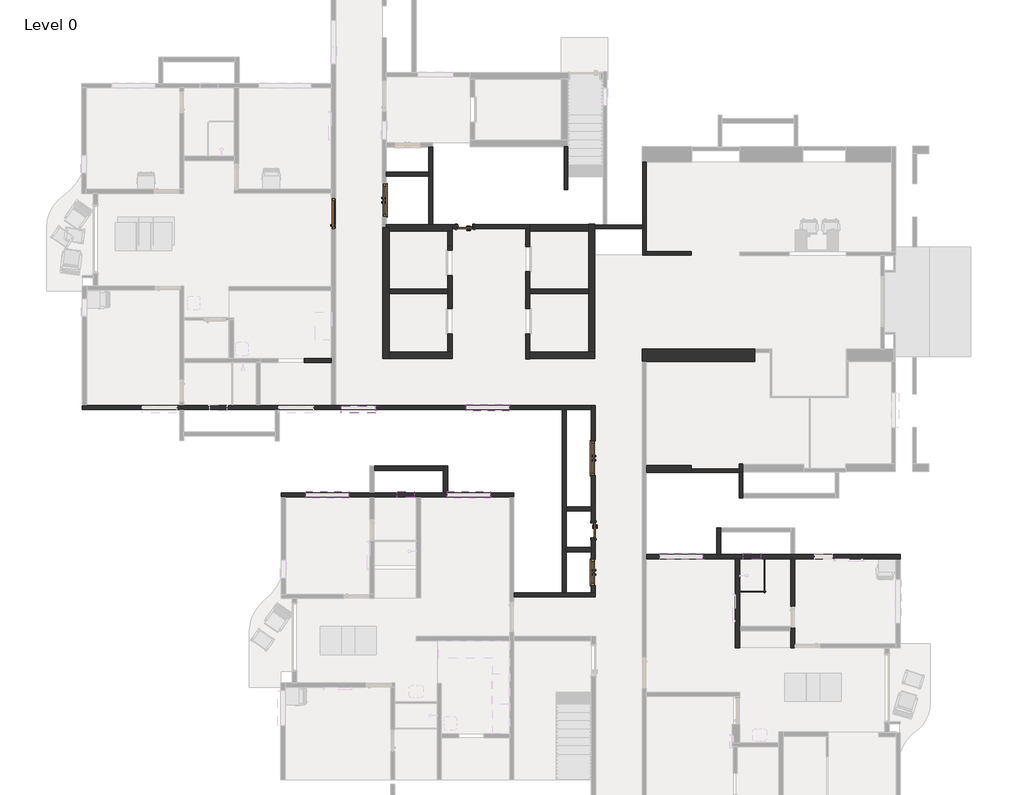
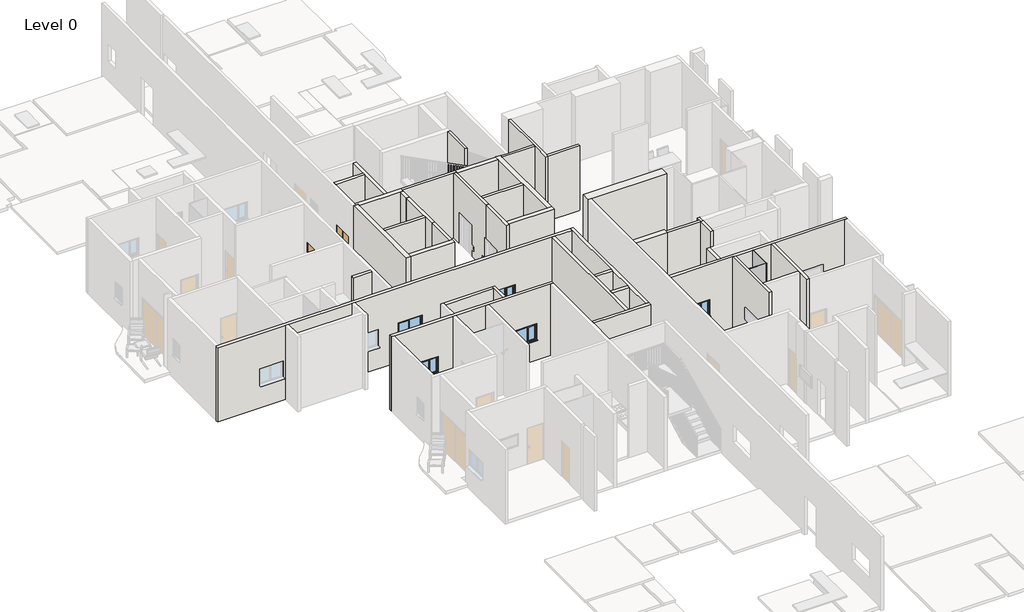
# One storey, part 5 of 14: 39 walls, 7 windows, 6 doors, 2 plates.
"""IFC4 building model written with IfcOpenShell, lengths in millimetres."""

from ifc_helpers import new_model, si_unit, origin, origin_with_axes, place, context, project, spatial, polyline, outline, extrude, faceted_brep, transform, mapped, element, save
from components import doors_extdbl_flush_3_b8e651f3, doors_extdbl_flush_3_75_39ca422f, doors_extdbl_flush_4_40db91a8, doors_extsgl_flush_d1_30a970b5, doors_intsgl_2_0e89f101, system_panel_glazed_234dce3e, system_panel_glazed_3e513c0f, windows_concept_plain_dbl_4_d1e2e333, windows_sgl_plain_2_be143095, windows_tpl_variable_casement_5_ffad3fa3

model = new_model("IFC4")

# Units and contexts
model_context = context("Model", 3, world=origin())
ifc_project = project(units=[si_unit("LENGTHUNIT", "METRE", prefix="MILLI")], contexts=[model_context])

# Site, building, storey
site = spatial("IfcSite", under=ifc_project)
building = spatial("IfcBuilding", under=site)
storey = spatial("IfcBuildingStorey", under=building, Name="Level 0", Elevation=0.0)

# Doors
placement = place(None, origin())
doors_extdbl_flush_3_shape = doors_extdbl_flush_3_b8e651f3(model_context)
element("IfcDoor", 1, ObjectType="Doors_ExtDbl_Flush : 3'", at=placement, inside=storey, context=model_context, shape_type="MappedRepresentation", body=[
    mapped(doors_extdbl_flush_3_shape, transform((-21675.1800447, 33308.7351384, 0.0), x_axis=(0.0, 1.0, 0.0), y_axis=(-1.0, 0.0, 0.0), z_axis=(0.0, 0.0, 1.0))),
])
doors_extdbl_flush_3_75_shape = doors_extdbl_flush_3_75_39ca422f(model_context)
element("IfcDoor", 2, ObjectType="Doors_ExtDbl_Flush : 3.75'", at=placement, inside=storey, context=model_context, shape_type="MappedRepresentation", body=[
    mapped(doors_extdbl_flush_3_75_shape, transform((-29094.6788109, 46525.3706597, 0.0), x_axis=(0.0, -1.0, 0.0), y_axis=(1.0, 0.0, 0.0), z_axis=(0.0, 0.0, 1.0))),
])
doors_extdbl_flush_4_shape = doors_extdbl_flush_4_40db91a8(model_context)
element("IfcDoor", 3, ObjectType="Doors_ExtDbl_Flush : 4'", at=placement, inside=storey, context=model_context, shape_type="MappedRepresentation", body=[
    mapped(doors_extdbl_flush_4_shape, transform((-21675.1800447, 37361.9567572, 0.0), x_axis=(0.0, 1.0, 0.0), y_axis=(-1.0, 0.0, 0.0), z_axis=(0.0, 0.0, 1.0))),
])
doors_extsgl_flush_d1_shape = doors_extsgl_flush_d1_30a970b5(model_context)
element("IfcDoor", 4, ObjectType="Doors_ExtSgl_Flush : D1", at=placement, inside=storey, context=model_context, shape_type="MappedRepresentation", body=[
    mapped(doors_extsgl_flush_d1_shape, transform((-30896.1442282, 46044.6966557, 0.0), x_axis=(0.0, 1.0, 0.0), y_axis=(-1.0, 0.0, 0.0), z_axis=(0.0, 0.0, 1.0))),
])
doors_intsgl_2_shape = doors_intsgl_2_0e89f101(model_context)
element("IfcDoor", 5, ObjectType="Doors_IntSgl : 2'", at=placement, inside=storey, context=model_context, shape_type="MappedRepresentation", body=[
    mapped(doors_intsgl_2_shape, transform((-21675.1800447, 34796.5704211, 0.0), x_axis=(0.0, -1.0, 0.0), y_axis=(1.0, 0.0, 0.0), z_axis=(0.0, 0.0, 1.0))),
])
element("IfcDoor", 6, ObjectType="Doors_IntSgl : 2'", at=placement, inside=storey, context=model_context, shape_type="MappedRepresentation", body=[
    mapped(doors_intsgl_2_shape, transform((-26226.4805211, 45585.4690597, 0.0), x_axis=(-1.0, 0.0, 0.0), y_axis=(0.0, -1.0, 0.0), z_axis=(0.0, 0.0, 1.0))),
])

# Plates
system_panel_glazed_shape = system_panel_glazed_234dce3e(model_context)
element("IfcPlate", 7, ObjectType="System Panel : Glazed", at=placement, inside=storey, context=model_context, shape_type="MappedRepresentation", body=[
    mapped(system_panel_glazed_shape, transform((-16019.2486976, 32586.7114683, 0.0), x_axis=(1.0, 0.0, 0.0), y_axis=(0.0, 1.0, 0.0), z_axis=(0.0, 0.0, 1.0))),
])
system_panel_glazed_2_shape = system_panel_glazed_3e513c0f(model_context)
element("IfcPlate", 8, ObjectType="System Panel : Glazed", at=placement, inside=storey, context=model_context, shape_type="MappedRepresentation", body=[
    mapped(system_panel_glazed_2_shape, transform((-15562.0486976, 33186.8118683, 0.0), x_axis=(0.0, 1.0, 0.0), y_axis=(-1.0, 0.0, 0.0), z_axis=(0.0, 0.0, 1.0))),
])

# Walls
element("IfcWall", 9, ObjectType="W1", at=placement, inside=storey, context=model_context, shape_type="Brep", body=[
    faceted_brep([(-24494.5800447, 36137.3800488, 0.0), (-26841.4029681, 36137.3800488, 0.0), (-26993.8029681, 36137.3800488, 0.0), (-29458.4489269, 36137.3800488, 0.0), (-29610.8489269, 36137.3800488, 0.0), (-32744.0041796, 36137.3800488, 0.0), (-32744.0041796, 36137.3800488, 4000.0), (-29610.8489269, 36137.3800488, 4000.0), (-29458.4489269, 36137.3800488, 4000.0), (-26993.8029681, 36137.3800488, 4000.0), (-26841.4029681, 36137.3800488, 4000.0), (-24494.5800447, 36137.3800488, 4000.0), (-26856.7800447, 36137.3800488, 2110.0), (-26856.7800447, 36137.3800488, 1200.0), (-25332.7800447, 36137.3800488, 1200.0), (-25332.7800447, 36137.3800488, 2110.0), (-31880.4041796, 36137.3800488, 2110.0), (-31880.4041796, 36137.3800488, 1200.0), (-30356.4041796, 36137.3800488, 1200.0), (-30356.4041796, 36137.3800488, 2110.0), (-28638.8447747, 36137.3800488, 2738.9328), (-28638.8447747, 36137.3800488, 1828.9328), (-28029.2447747, 36137.3800488, 1828.9328), (-28029.2447747, 36137.3800488, 2738.9328), (-24494.5800447, 35984.9800488, 0.0), (-24494.5800447, 35984.9800488, 4000.0), (-24646.9800447, 35984.9800488, 4000.0), (-27800.6447747, 35984.9800488, 4000.0), (-27953.0447747, 35984.9800488, 4000.0), (-29458.4489269, 35984.9800488, 4000.0), (-29610.8489269, 35984.9800488, 4000.0), (-32591.6041796, 35984.9800488, 4000.0), (-32744.0041796, 35984.9800488, 4000.0), (-32744.0041796, 35984.9800488, 0.0), (-32591.6041796, 35984.9800488, 0.0), (-29610.8489269, 35984.9800488, 0.0), (-29458.4489269, 35984.9800488, 0.0), (-27953.0447747, 35984.9800488, 0.0), (-27800.6447747, 35984.9800488, 0.0), (-24646.9800447, 35984.9800488, 0.0), (-26856.7800447, 35984.9800488, 2110.0), (-25332.7800447, 35984.9800488, 2110.0), (-25332.7800447, 35984.9800488, 1200.0), (-26856.7800447, 35984.9800488, 1200.0), (-31880.4041796, 35984.9800488, 2110.0), (-30356.4041796, 35984.9800488, 2110.0), (-30356.4041796, 35984.9800488, 1200.0), (-31880.4041796, 35984.9800488, 1200.0), (-28638.8447747, 35984.9800488, 2738.9328), (-28029.2447747, 35984.9800488, 2738.9328), (-28029.2447747, 35984.9800488, 1828.9328), (-28638.8447747, 35984.9800488, 1828.9328)], [[[0, 1, 2, 3, 4, 5, 6, 7, 8, 9, 10, 11], [12, 13, 14, 15], [16, 17, 18, 19], [20, 21, 22, 23]], [[24, 25, 26, 27, 28, 29, 30, 31, 32, 33, 34, 35, 36, 37, 38, 39], [40, 41, 42, 43], [44, 45, 46, 47], [48, 49, 50, 51]], [[5, 4, 3, 2, 1, 0, 24, 39, 38, 37, 36, 35, 34, 33]], [[11, 10, 9, 8, 7, 6, 32, 31, 30, 29, 28, 27, 26, 25]], [[6, 5, 33, 32]], [[0, 11, 25, 24]], [[13, 12, 40, 43]], [[14, 13, 43, 42]], [[15, 14, 42, 41]], [[12, 15, 41, 40]], [[17, 16, 44, 47]], [[18, 17, 47, 46]], [[19, 18, 46, 45]], [[16, 19, 45, 44]], [[21, 20, 48, 51]], [[22, 21, 51, 50]], [[23, 22, 50, 49]], [[20, 23, 49, 48]]]),
])
element("IfcWall", 10, ObjectType="W1", at=placement, inside=storey, context=model_context, shape_type="Brep", body=[
    faceted_brep([(-19793.4917798, 33786.9122683, 0.0), (-16628.8486976, 33786.9122683, 0.0), (-16476.4486976, 33786.9122683, 0.0), (-14673.0486976, 33786.9122683, 0.0), (-14520.6486976, 33786.9122683, 0.0), (-10935.2417798, 33786.9122683, 0.0), (-10782.8417798, 33786.9122683, 0.0), (-10782.8417798, 33786.9122683, 4000.0), (-10935.2417798, 33786.9122683, 4000.0), (-14520.6486976, 33786.9122683, 4000.0), (-14673.0486976, 33786.9122683, 4000.0), (-16476.4486976, 33786.9122683, 4000.0), (-16628.8486976, 33786.9122683, 4000.0), (-19793.4917798, 33786.9122683, 4000.0), (-19309.7710387, 33786.9122683, 2110.0), (-17785.7710387, 33786.9122683, 2110.0), (-17785.7710387, 33786.9122683, 1200.0), (-19309.7710387, 33786.9122683, 1200.0), (-16349.4486976, 33786.9122683, 2738.9328), (-15739.8486976, 33786.9122683, 2738.9328), (-15739.8486976, 33786.9122683, 1828.9328), (-16349.4486976, 33786.9122683, 1828.9328), (-13809.4486976, 33786.9122683, 2110.0), (-13199.8486976, 33786.9122683, 2110.0), (-13199.8486976, 33786.9122683, 1200.0), (-13809.4486976, 33786.9122683, 1200.0), (-19793.4917798, 33939.3122683, 0.0), (-19793.4917798, 33939.3122683, 4000.0), (-17302.0502976, 33939.3122683, 4000.0), (-17149.6502976, 33939.3122683, 4000.0), (-14673.0486976, 33939.3122683, 4000.0), (-14520.6486976, 33939.3122683, 4000.0), (-10782.8417798, 33939.3122683, 4000.0), (-10782.8417798, 33939.3122683, 0.0), (-14520.6486976, 33939.3122683, 0.0), (-14673.0486976, 33939.3122683, 0.0), (-17149.6502976, 33939.3122683, 0.0), (-17302.0502976, 33939.3122683, 0.0), (-19309.7710387, 33939.3122683, 2110.0), (-19309.7710387, 33939.3122683, 1200.0), (-17785.7710387, 33939.3122683, 1200.0), (-17785.7710387, 33939.3122683, 2110.0), (-16349.4486976, 33939.3122683, 2738.9328), (-16349.4486976, 33939.3122683, 1828.9328), (-15739.8486976, 33939.3122683, 1828.9328), (-15739.8486976, 33939.3122683, 2738.9328), (-13809.4486976, 33939.3122683, 2110.0), (-13809.4486976, 33939.3122683, 1200.0), (-13199.8486976, 33939.3122683, 1200.0), (-13199.8486976, 33939.3122683, 2110.0)], [[[0, 1, 2, 3, 4, 5, 6, 7, 8, 9, 10, 11, 12, 13], [14, 15, 16, 17], [18, 19, 20, 21], [22, 23, 24, 25]], [[26, 27, 28, 29, 30, 31, 32, 33, 34, 35, 36, 37], [38, 39, 40, 41], [42, 43, 44, 45], [46, 47, 48, 49]], [[6, 5, 4, 3, 2, 1, 0, 26, 37, 36, 35, 34, 33]], [[13, 12, 11, 10, 9, 8, 7, 32, 31, 30, 29, 28, 27]], [[0, 13, 27, 26]], [[7, 6, 33, 32]], [[39, 38, 14, 17]], [[40, 39, 17, 16]], [[41, 40, 16, 15]], [[38, 41, 15, 14]], [[43, 42, 18, 21]], [[44, 43, 21, 20]], [[45, 44, 20, 19]], [[42, 45, 19, 18]], [[47, 46, 22, 25]], [[48, 47, 25, 24]], [[49, 48, 24, 23]], [[46, 49, 23, 22]]]),
])
element("IfcWall", 11, ObjectType="W1", at=placement, inside=storey, context=model_context, shape_type="Brep", body=[
    faceted_brep([(-17302.0502976, 34891.8759386, 0.0), (-17302.0502976, 33939.3122683, 0.0), (-17302.0502976, 33939.3122683, 4000.0), (-17302.0502976, 34891.8759386, 4000.0), (-17149.6502976, 34891.8759386, 0.0), (-17149.6502976, 34891.8759386, 4000.0), (-17149.6502976, 34739.4759386, 4000.0), (-17149.6502976, 33939.3122683, 4000.0), (-17149.6502976, 33939.3122683, 0.0), (-17149.6502976, 34739.4759386, 0.0)], [[[0, 1, 2, 3]], [[4, 5, 6, 7, 8, 9]], [[1, 0, 4, 9, 8]], [[3, 2, 7, 6, 5]], [[2, 1, 8, 7]], [[0, 3, 5, 4]]]),
])
element("IfcWall", 12, ObjectType="W1", at=placement, inside=storey, context=model_context, shape_type="Brep", body=[
    faceted_brep([(-14673.0486976, 31335.7106683, 2110.0), (-14673.0486976, 31335.7106683, 0.0), (-14673.0486976, 31234.1106683, 0.0), (-14673.0486976, 30624.5106683, 0.0), (-14673.0486976, 30624.5106683, 4000.0), (-14673.0486976, 31234.1106683, 4000.0), (-14673.0486976, 31386.5106683, 4000.0), (-14673.0486976, 33786.9122683, 4000.0), (-14673.0486976, 33786.9122683, 0.0), (-14673.0486976, 32097.7106683, 0.0), (-14673.0486976, 32097.7106683, 2110.0), (-14520.6486976, 30776.9106683, 0.0), (-14520.6486976, 31335.7106683, 0.0), (-14520.6486976, 31335.7106683, 2110.0), (-14520.6486976, 32097.7106683, 2110.0), (-14520.6486976, 32097.7106683, 0.0), (-14520.6486976, 33786.9122683, 0.0), (-14520.6486976, 33786.9122683, 4000.0), (-14520.6486976, 30776.9106683, 4000.0), (-14520.6486976, 30624.5106683, 4000.0), (-14520.6486976, 30624.5106683, 2110.0), (-14520.6486976, 30776.9106683, 2110.0), (-14546.0486976, 30776.9106683, 0.0), (-14546.0486976, 30624.5106683, 0.0), (-14546.0486976, 30624.5106683, 2110.0), (-14546.0486976, 30776.9106683, 2110.0)], [[[0, 1, 2, 3, 4, 5, 6, 7, 8, 9, 10]], [[11, 12, 13, 14, 15, 16, 17, 18, 19, 20, 21]], [[9, 8, 16, 15]], [[3, 2, 1, 12, 11, 22, 23]], [[7, 6, 5, 4, 19, 18, 17]], [[8, 7, 17, 16]], [[4, 3, 23, 24, 20, 19]], [[25, 22, 11, 21]], [[22, 25, 24, 23]], [[24, 25, 21, 20]], [[15, 14, 10, 9]], [[13, 12, 1, 0]], [[14, 13, 0, 10]]]),
])
element("IfcWall", 13, ObjectType="W1", at=placement, inside=storey, context=model_context, shape_type="Brep", body=[
    faceted_brep([(-16628.8486976, 33786.9122683, 0.0), (-16628.8486976, 30624.5106683, 0.0), (-16628.8486976, 30624.5106683, 4000.0), (-16628.8486976, 33786.9122683, 4000.0), (-16476.4486976, 33786.9122683, 0.0), (-16476.4486976, 33786.9122683, 4000.0), (-16476.4486976, 31386.5106683, 4000.0), (-16476.4486976, 31234.1106683, 4000.0), (-16476.4486976, 30624.5106683, 4000.0), (-16476.4486976, 30624.5106683, 0.0), (-16476.4486976, 31234.1106683, 0.0), (-16476.4486976, 31386.5106683, 0.0)], [[[0, 1, 2, 3]], [[4, 5, 6, 7, 8, 9, 10, 11]], [[1, 0, 4, 11, 10, 9]], [[2, 1, 9, 8]], [[3, 2, 8, 7, 6, 5]], [[0, 3, 5, 4]]]),
])
element("IfcWall", 14, ObjectType="W1", at=placement, inside=storey, context=model_context, shape_type="Brep", body=[
    faceted_brep([(-26841.4029681, 36137.3800488, 0.0), (-26841.4029681, 37081.0541094, 0.0), (-26841.4029681, 37081.0541094, 4000.0), (-26841.4029681, 36137.3800488, 4000.0), (-26993.8029681, 36137.3800488, 0.0), (-26993.8029681, 36137.3800488, 4000.0), (-26993.8029681, 36928.6541094, 4000.0), (-26993.8029681, 37081.0541094, 4000.0), (-26993.8029681, 37081.0541094, 0.0), (-26993.8029681, 36928.6541094, 0.0)], [[[0, 1, 2, 3]], [[4, 5, 6, 7, 8, 9]], [[1, 0, 4, 9, 8]], [[3, 2, 7, 6, 5]], [[0, 3, 5, 4]], [[2, 1, 8, 7]]]),
])
element("IfcWall", 15, ObjectType="W1", at=placement, inside=storey, context=model_context, shape_type="Brep", body=[
    faceted_brep([(-24494.5800447, 32430.4998557, 0.0), (-21598.9800447, 32430.4998557, 0.0), (-21598.9800447, 32430.4998557, 4000.0), (-24494.5800447, 32430.4998557, 4000.0), (-24494.5800447, 32582.8998557, 0.0), (-24494.5800447, 32582.8998557, 4000.0), (-22780.1816447, 32582.8998557, 4000.0), (-22627.7816447, 32582.8998557, 4000.0), (-21751.3800447, 32582.8998557, 4000.0), (-21598.9800447, 32582.8998557, 4000.0), (-21598.9800447, 32582.8998557, 0.0), (-21751.3800447, 32582.8998557, 0.0), (-22627.7816447, 32582.8998557, 0.0), (-22780.1816447, 32582.8998557, 0.0)], [[[0, 1, 2, 3]], [[4, 5, 6, 7, 8, 9, 10, 11, 12, 13]], [[1, 0, 4, 13, 12, 11, 10]], [[3, 2, 9, 8, 7, 6, 5]], [[0, 3, 5, 4]], [[2, 1, 10, 9]]]),
])
element("IfcWall", 16, ObjectType="W1", at=placement, inside=storey, context=model_context, shape_type="Brep", body=[
    faceted_brep([(-21598.9800447, 39237.6998557, 4000.0), (-21598.9800447, 32582.8998557, 4000.0), (-21598.9800447, 32582.8998557, 0.0), (-21598.9800447, 32851.5351384, 0.0), (-21598.9800447, 32851.5351384, 2110.0), (-21598.9800447, 33765.9351384, 2110.0), (-21598.9800447, 33765.9351384, 0.0), (-21598.9800447, 34491.7704211, 0.0), (-21598.9800447, 34491.7704211, 2110.0), (-21598.9800447, 35101.3704211, 2110.0), (-21598.9800447, 35101.3704211, 0.0), (-21598.9800447, 36752.3567572, 0.0), (-21598.9800447, 36752.3567572, 2110.0), (-21598.9800447, 37971.5567572, 2110.0), (-21598.9800447, 37971.5567572, 0.0), (-21598.9800447, 39237.6998557, 0.0), (-21751.3800447, 32582.8998557, 4000.0), (-21751.3800447, 34034.5704211, 4000.0), (-21751.3800447, 34186.9704211, 4000.0), (-21751.3800447, 35486.2136587, 4000.0), (-21751.3800447, 35638.6136587, 4000.0), (-21751.3800447, 39085.2998557, 4000.0), (-21751.3800447, 39237.6998557, 4000.0), (-21751.3800447, 39237.6998557, 0.0), (-21751.3800447, 39085.2998557, 0.0), (-21751.3800447, 37971.5567572, 0.0), (-21751.3800447, 37971.5567572, 2110.0), (-21751.3800447, 36752.3567572, 2110.0), (-21751.3800447, 36752.3567572, 0.0), (-21751.3800447, 35638.6136587, 0.0), (-21751.3800447, 35486.2136587, 0.0), (-21751.3800447, 35101.3704211, 0.0), (-21751.3800447, 35101.3704211, 2110.0), (-21751.3800447, 34491.7704211, 2110.0), (-21751.3800447, 34491.7704211, 0.0), (-21751.3800447, 34186.9704211, 0.0), (-21751.3800447, 34034.5704211, 0.0), (-21751.3800447, 33765.9351384, 0.0), (-21751.3800447, 33765.9351384, 2110.0), (-21751.3800447, 32851.5351384, 2110.0), (-21751.3800447, 32851.5351384, 0.0), (-21751.3800447, 32582.8998557, 0.0)], [[[0, 1, 2, 3, 4, 5, 6, 7, 8, 9, 10, 11, 12, 13, 14, 15]], [[16, 17, 18, 19, 20, 21, 22, 23, 24, 25, 26, 27, 28, 29, 30, 31, 32, 33, 34, 35, 36, 37, 38, 39, 40, 41]], [[2, 41, 40, 3]], [[23, 15, 14, 25, 24]], [[28, 11, 10, 31, 30, 29]], [[6, 37, 36, 35, 34, 7]], [[1, 0, 22, 21, 20, 19, 18, 17, 16]], [[2, 1, 16, 41]], [[0, 15, 23, 22]], [[28, 27, 12, 11]], [[26, 25, 14, 13]], [[27, 26, 13, 12]], [[40, 39, 4, 3]], [[38, 37, 6, 5]], [[39, 38, 5, 4]], [[33, 8, 7, 34]], [[8, 33, 32, 9]], [[9, 32, 31, 10]]]),
])
element("IfcWall", 17, ObjectType="W1", at=placement, inside=storey, context=model_context, shape_type="Brep", body=[
    faceted_brep([(-22627.7816447, 32582.8998557, 0.0), (-22627.7816447, 34034.5704211, 0.0), (-22627.7816447, 34186.9704211, 0.0), (-22627.7816447, 35486.2136587, 0.0), (-22627.7816447, 35638.6136587, 0.0), (-22627.7816447, 39085.2998557, 0.0), (-22627.7816447, 39085.2998557, 4000.0), (-22627.7816447, 35638.6136587, 4000.0), (-22627.7816447, 35486.2136587, 4000.0), (-22627.7816447, 34186.9704211, 4000.0), (-22627.7816447, 34034.5704211, 4000.0), (-22627.7816447, 32582.8998557, 4000.0), (-22780.1816447, 32582.8998557, 0.0), (-22780.1816447, 32582.8998557, 4000.0), (-22780.1816447, 39085.2998557, 4000.0), (-22780.1816447, 39085.2998557, 0.0)], [[[0, 1, 2, 3, 4, 5, 6, 7, 8, 9, 10, 11]], [[12, 13, 14, 15]], [[5, 4, 3, 2, 1, 0, 12, 15]], [[11, 10, 9, 8, 7, 6, 14, 13]], [[0, 11, 13, 12]], [[6, 5, 15, 14]]]),
])
element("IfcWall", 18, ObjectType="W1", at=placement, inside=storey, context=model_context, shape_type="Brep", body=[
    faceted_brep([(-21751.3800447, 39237.6998557, 0.0), (-30819.9442282, 39237.6998557, 0.0), (-30972.3442282, 39237.6998557, 0.0), (-33487.7823022, 39237.6998557, 0.0), (-33640.1823022, 39237.6998557, 0.0), (-36205.5823022, 39237.6998557, 0.0), (-36357.9823022, 39237.6998557, 0.0), (-39658.4816447, 39237.6998557, 0.0), (-39810.8816447, 39237.6998557, 0.0), (-39810.8816447, 39237.6998557, 4000.0), (-39658.4816447, 39237.6998557, 4000.0), (-36357.9823022, 39237.6998557, 4000.0), (-36205.5823022, 39237.6998557, 4000.0), (-33640.1823022, 39237.6998557, 4000.0), (-33487.7823022, 39237.6998557, 4000.0), (-30972.3442282, 39237.6998557, 4000.0), (-30819.9442282, 39237.6998557, 4000.0), (-21751.3800447, 39237.6998557, 4000.0), (-31620.4632652, 39237.6998557, 2110.0), (-32839.6632652, 39237.6998557, 2110.0), (-32839.6632652, 39237.6998557, 1200.0), (-31620.4632652, 39237.6998557, 1200.0), (-36458.0816447, 39237.6998557, 2110.0), (-37677.2816447, 39237.6998557, 2110.0), (-37677.2816447, 39237.6998557, 1200.0), (-36458.0816447, 39237.6998557, 1200.0), (-34681.5823022, 39237.6998557, 2738.9328), (-35291.1823022, 39237.6998557, 2738.9328), (-35291.1823022, 39237.6998557, 1828.9328), (-34681.5823022, 39237.6998557, 1828.9328), (-29397.5442282, 39237.6998557, 2110.0), (-30616.7442282, 39237.6998557, 2110.0), (-30616.7442282, 39237.6998557, 1200.0), (-29397.5442282, 39237.6998557, 1200.0), (-24659.7816447, 39237.6998557, 2110.0), (-26183.7816447, 39237.6998557, 2110.0), (-26183.7816447, 39237.6998557, 1200.0), (-24659.7816447, 39237.6998557, 1200.0), (-21751.3800447, 39085.2998557, 0.0), (-21751.3800447, 39085.2998557, 4000.0), (-22627.7816447, 39085.2998557, 4000.0), (-22780.1816447, 39085.2998557, 4000.0), (-32813.1816447, 39085.2998557, 4000.0), (-32965.5816447, 39085.2998557, 4000.0), (-36205.5823022, 39085.2998557, 4000.0), (-36357.9823022, 39085.2998557, 4000.0), (-39810.8816447, 39085.2998557, 4000.0), (-39810.8816447, 39085.2998557, 0.0), (-36357.9823022, 39085.2998557, 0.0), (-36205.5823022, 39085.2998557, 0.0), (-32965.5816447, 39085.2998557, 0.0), (-32813.1816447, 39085.2998557, 0.0), (-22780.1816447, 39085.2998557, 0.0), (-22627.7816447, 39085.2998557, 0.0), (-31620.4632652, 39085.2998557, 2110.0), (-31620.4632652, 39085.2998557, 1200.0), (-32839.6632652, 39085.2998557, 1200.0), (-32839.6632652, 39085.2998557, 2110.0), (-36458.0816447, 39085.2998557, 2110.0), (-36458.0816447, 39085.2998557, 1200.0), (-37677.2816447, 39085.2998557, 1200.0), (-37677.2816447, 39085.2998557, 2110.0), (-34681.5823022, 39085.2998557, 2738.9328), (-34681.5823022, 39085.2998557, 1828.9328), (-35291.1823022, 39085.2998557, 1828.9328), (-35291.1823022, 39085.2998557, 2738.9328), (-29397.5442282, 39085.2998557, 2110.0), (-29397.5442282, 39085.2998557, 1200.0), (-30616.7442282, 39085.2998557, 1200.0), (-30616.7442282, 39085.2998557, 2110.0), (-24659.7816447, 39085.2998557, 2110.0), (-24659.7816447, 39085.2998557, 1200.0), (-26183.7816447, 39085.2998557, 1200.0), (-26183.7816447, 39085.2998557, 2110.0)], [[[0, 1, 2, 3, 4, 5, 6, 7, 8, 9, 10, 11, 12, 13, 14, 15, 16, 17], [18, 19, 20, 21], [22, 23, 24, 25], [26, 27, 28, 29], [30, 31, 32, 33], [34, 35, 36, 37]], [[38, 39, 40, 41, 42, 43, 44, 45, 46, 47, 48, 49, 50, 51, 52, 53], [54, 55, 56, 57], [58, 59, 60, 61], [62, 63, 64, 65], [66, 67, 68, 69], [70, 71, 72, 73]], [[8, 7, 6, 5, 4, 3, 2, 1, 0, 38, 53, 52, 51, 50, 49, 48, 47]], [[17, 16, 15, 14, 13, 12, 11, 10, 9, 46, 45, 44, 43, 42, 41, 40, 39]], [[0, 17, 39, 38]], [[9, 8, 47, 46]], [[55, 54, 18, 21]], [[56, 55, 21, 20]], [[57, 56, 20, 19]], [[54, 57, 19, 18]], [[59, 58, 22, 25]], [[60, 59, 25, 24]], [[61, 60, 24, 23]], [[58, 61, 23, 22]], [[63, 62, 26, 29]], [[64, 63, 29, 28]], [[65, 64, 28, 27]], [[62, 65, 27, 26]], [[67, 66, 30, 33]], [[68, 67, 33, 32]], [[69, 68, 32, 31]], [[66, 69, 31, 30]], [[71, 70, 34, 37]], [[72, 71, 37, 36]], [[73, 72, 36, 35]], [[70, 73, 35, 34]]]),
])
element("IfcWall", 19, ObjectType="W1", at=placement, inside=storey, context=model_context, shape_type="SweptSolid", body=[
    extrude(outline(polyline([(-22627.7816447, 35638.6136587), (-21751.3800447, 35638.6136587), (-21751.3800447, 35486.2136587), (-22627.7816447, 35486.2136587), (-22627.7816447, 35638.6136587)])), origin_with_axes(), (0.0, 0.0, 1.0), 4000.0),
])
element("IfcWall", 20, ObjectType="W1", at=placement, inside=storey, context=model_context, shape_type="SweptSolid", body=[
    extrude(outline(polyline([(-22627.7816447, 34186.9704211), (-21751.3800447, 34186.9704211), (-21751.3800447, 34034.5704211), (-22627.7816447, 34034.5704211), (-22627.7816447, 34186.9704211)])), origin_with_axes(), (0.0, 0.0, 1.0), 4000.0),
])
element("IfcWall", 21, ObjectType="W1", at=placement, inside=storey, context=model_context, shape_type="Brep", body=[
    faceted_brep([(-27519.7772109, 48417.6706597, 0.0), (-27519.7772109, 47528.6706597, 0.0), (-27519.7772109, 47376.2706597, 0.0), (-27519.7772109, 45661.6690597, 0.0), (-27519.7772109, 45661.6690597, 4000.0), (-27519.7772109, 47376.2706597, 4000.0), (-27519.7772109, 47528.6706597, 4000.0), (-27519.7772109, 48417.6706597, 4000.0), (-27367.3772109, 48417.6706597, 0.0), (-27367.3772109, 48417.6706597, 4000.0), (-27367.3772109, 45661.6690597, 4000.0), (-27367.3772109, 45661.6690597, 0.0)], [[[0, 1, 2, 3, 4, 5, 6, 7]], [[8, 9, 10, 11]], [[3, 2, 1, 0, 8, 11]], [[7, 6, 5, 4, 10, 9]], [[0, 7, 9, 8]], [[4, 3, 11, 10]]]),
])
element("IfcWall", 22, ObjectType="W1", at=placement, inside=storey, context=model_context, shape_type="SweptSolid", body=[
    extrude(outline(polyline([(-27519.7772109, 47376.2706597), (-29018.4788109, 47376.2706597), (-29018.4788109, 47528.6706597), (-27519.7772109, 47528.6706597), (-27519.7772109, 47376.2706597)])), origin_with_axes(), (0.0, 0.0, 1.0), 4000.0),
])
element("IfcWall", 23, ObjectType="W1", at=placement, inside=storey, context=model_context, shape_type="Brep", body=[
    faceted_brep([(-26683.6805211, 42677.5183335, 4000.0), (-26683.6805211, 41129.4738327, 4000.0), (-26683.6805211, 41129.4738327, 0.0), (-26683.6805211, 41777.5183335, 0.0), (-26683.6805211, 41777.5183335, 2100.0), (-26683.6805211, 42677.5183335, 2100.0), (-26836.0805211, 41129.4738327, 4000.0), (-26836.0805211, 42677.5183335, 4000.0), (-26836.0805211, 42677.5183335, 2100.0), (-26836.0805211, 41777.5183335, 2100.0), (-26836.0805211, 41777.5183335, 0.0), (-26836.0805211, 41129.4738327, 0.0), (-26686.0514993, 42677.5183335, 4000.0)], [[[0, 1, 2, 3, 4, 5]], [[6, 7, 8, 9, 10, 11]], [[2, 11, 10, 3]], [[7, 12, 0, 5, 8]], [[1, 0, 12, 7, 6]], [[2, 1, 6, 11]], [[4, 9, 8, 5]], [[9, 4, 3, 10]]]),
])
element("IfcWall", 24, ObjectType="W1", at=placement, inside=storey, context=model_context, shape_type="Brep", body=[
    faceted_brep([(-26686.0514993, 44899.6690597, 0.0), (-26686.0514993, 44899.6690597, 4000.0), (-26686.0514993, 42677.5183335, 4000.0), (-26686.0514993, 42677.5183335, 0.0), (-26686.0514993, 43847.2690597, 0.0), (-26686.0514993, 43847.2690597, 2100.0), (-26686.0514993, 44747.2690597, 2100.0), (-26686.0514993, 44747.2690597, 0.0), (-26838.4514993, 44899.6690597, 4000.0), (-26838.4514993, 44899.6690597, 0.0), (-26838.4514993, 44747.2690597, 0.0), (-26838.4514993, 44747.2690597, 2100.0), (-26838.4514993, 43847.2690597, 2100.0), (-26838.4514993, 43847.2690597, 0.0), (-26838.4514993, 43363.3183335, 0.0), (-26838.4514993, 43210.9183335, 0.0), (-26838.4514993, 42677.5183335, 0.0), (-26838.4514993, 42677.5183335, 4000.0), (-26838.4514993, 43210.9183335, 4000.0), (-26838.4514993, 43363.3183335, 4000.0), (-26836.0805211, 44899.6690597, 0.0), (-26836.0805211, 44899.6690597, 4000.0), (-26836.0805211, 42677.5183335, 4000.0)], [[[0, 1, 2, 3, 4, 5, 6, 7]], [[8, 9, 10, 11, 12, 13, 14, 15, 16, 17, 18, 19]], [[3, 16, 15, 14, 13, 4]], [[9, 20, 0, 7, 10]], [[1, 0, 20, 9, 8, 21]], [[2, 1, 21, 8, 19, 18, 17, 22]], [[3, 2, 22, 17, 16]], [[6, 11, 10, 7]], [[11, 6, 5, 12]], [[12, 5, 4, 13]]]),
])
element("IfcWall", 25, ObjectType="W1", at=placement, inside=storey, context=model_context, shape_type="Brep", body=[
    faceted_brep([(-26683.6805211, 44899.6690597, 0.0), (-26683.6805211, 45433.0690597, 0.0), (-26683.6805211, 45433.0690597, 4000.0), (-26683.6805211, 44899.6690597, 4000.0), (-26836.0805211, 44899.6690597, 0.0), (-26836.0805211, 44899.6690597, 4000.0), (-26836.0805211, 45433.0690597, 4000.0), (-26836.0805211, 45433.0690597, 0.0), (-26686.0514993, 44899.6690597, 0.0), (-26686.0514993, 44899.6690597, 4000.0)], [[[0, 1, 2, 3]], [[4, 5, 6, 7]], [[1, 0, 8, 4, 7]], [[3, 2, 6, 5, 9]], [[0, 3, 9, 5, 4, 8]], [[2, 1, 7, 6]]]),
])
element("IfcWall", 26, ObjectType="W1", at=placement, inside=storey, context=model_context, shape_type="SweptSolid", body=[
    extrude(outline(polyline([(-26838.4514993, 43210.9183335), (-28918.8805211, 43210.9183335), (-28918.8805211, 43363.3183335), (-26838.4514993, 43363.3183335), (-26838.4514993, 43210.9183335)])), origin_with_axes(), (0.0, 0.0, 1.0), 4000.0),
])
element("IfcWall", 27, ObjectType="W1", at=placement, inside=storey, context=model_context, shape_type="Brep", body=[
    faceted_brep([(-23927.7805211, 45509.2690597, 4000.0), (-24080.1805211, 45509.2690597, 4000.0), (-26683.6805211, 45509.2690597, 4000.0), (-26683.6805211, 45509.2690597, 0.0), (-26531.2805211, 45509.2690597, 0.0), (-26531.2805211, 45509.2690597, 2110.0), (-25921.6805211, 45509.2690597, 2110.0), (-25921.6805211, 45509.2690597, 0.0), (-24080.1805211, 45509.2690597, 0.0), (-23927.7805211, 45509.2690597, 0.0), (-26683.6805211, 45661.6690597, 4000.0), (-23927.7805211, 45661.6690597, 4000.0), (-23927.7805211, 45661.6690597, 0.0), (-25921.6805211, 45661.6690597, 0.0), (-25921.6805211, 45661.6690597, 2110.0), (-26531.2805211, 45661.6690597, 2110.0), (-26531.2805211, 45661.6690597, 0.0), (-26683.6805211, 45661.6690597, 0.0)], [[[0, 1, 2, 3, 4, 5, 6, 7, 8, 9]], [[10, 11, 12, 13, 14, 15, 16, 17]], [[3, 17, 16, 4]], [[12, 9, 8, 7, 13]], [[2, 1, 0, 11, 10]], [[3, 2, 10, 17]], [[0, 9, 12, 11]], [[15, 5, 4, 16]], [[5, 15, 14, 6]], [[6, 14, 13, 7]]]),
])
element("IfcWall", 28, ObjectType="W1", at=placement, inside=storey, context=model_context, shape_type="Brep", body=[
    faceted_brep([(-24080.1805211, 42677.5183335, 0.0), (-24080.1805211, 42677.5183335, 4000.0), (-24080.1805211, 45509.2690597, 4000.0), (-24080.1805211, 45509.2690597, 0.0), (-24080.1805211, 44886.2936966, 0.0), (-24080.1805211, 44886.2936966, 2100.0), (-24080.1805211, 43986.2936966, 2100.0), (-24080.1805211, 43986.2936966, 0.0), (-23927.7805211, 42677.5183335, 4000.0), (-23927.7805211, 42677.5183335, 0.0), (-23927.7805211, 43210.9183335, 0.0), (-23927.7805211, 43363.3183335, 0.0), (-23927.7805211, 43986.2936966, 0.0), (-23927.7805211, 43986.2936966, 2100.0), (-23927.7805211, 44886.2936966, 2100.0), (-23927.7805211, 44886.2936966, 0.0), (-23927.7805211, 45433.0690597, 0.0), (-23927.7805211, 45509.2690597, 0.0), (-23927.7805211, 45509.2690597, 4000.0), (-23927.7805211, 45433.0690597, 4000.0), (-23927.7805211, 43363.3183335, 4000.0), (-23927.7805211, 43210.9183335, 4000.0), (-24078.3411875, 42677.5183335, 4000.0)], [[[0, 1, 2, 3, 4, 5, 6, 7]], [[8, 9, 10, 11, 12, 13, 14, 15, 16, 17, 18, 19, 20, 21]], [[9, 0, 7, 12, 11, 10]], [[3, 17, 16, 15, 4]], [[1, 0, 9, 8, 22]], [[2, 1, 22, 8, 21, 20, 19, 18]], [[3, 2, 18, 17]], [[14, 5, 4, 15]], [[5, 14, 13, 6]], [[6, 13, 12, 7]]]),
])
element("IfcWall", 29, ObjectType="W1", at=placement, inside=storey, context=model_context, shape_type="SweptSolid", body=[
    extrude(outline(polyline([(-21844.9805211, 43210.9183335), (-23927.7805211, 43210.9183335), (-23927.7805211, 43363.3183335), (-21844.9805211, 43363.3183335), (-21844.9805211, 43210.9183335)])), origin_with_axes(), (0.0, 0.0, 1.0), 4000.0),
])
element("IfcWall", 30, ObjectType="W1", at=placement, inside=storey, context=model_context, shape_type="Brep", body=[
    faceted_brep([(-24078.3411875, 40878.9954914, 0.0), (-24078.3411875, 40878.9954914, 4000.0), (-24078.3411875, 42677.5183335, 4000.0), (-24078.3411875, 42677.5183335, 2100.0), (-24078.3411875, 41777.5183335, 2100.0), (-24078.3411875, 41777.5183335, 0.0), (-23925.9411875, 40878.9954914, 4000.0), (-23925.9411875, 40878.9954914, 0.0), (-23925.9411875, 40904.3954914, 0.0), (-23925.9411875, 41132.9954914, 0.0), (-23925.9411875, 41777.5183335, 0.0), (-23925.9411875, 41777.5183335, 2100.0), (-23925.9411875, 42677.5183335, 2100.0), (-23925.9411875, 42677.5183335, 4000.0), (-23925.9411875, 41132.9954914, 4000.0), (-23925.9411875, 40904.3954914, 4000.0), (-23927.7805211, 42677.5183335, 4000.0)], [[[0, 1, 2, 3, 4, 5]], [[6, 7, 8, 9, 10, 11, 12, 13, 14, 15]], [[7, 0, 5, 10, 9, 8]], [[1, 0, 7, 6]], [[2, 1, 6, 15, 14, 13, 16]], [[2, 16, 13, 12, 3]], [[4, 11, 10, 5]], [[11, 4, 3, 12]]]),
])
element("IfcWall", 31, ObjectType="W1", at=placement, inside=storey, context=model_context, shape_type="SweptSolid", body=[
    extrude(outline(polyline([(-31937.5442282, 40908.6978471), (-30972.3442282, 40908.6978471), (-30972.3442282, 40756.2978471), (-31937.5442282, 40756.2978471), (-31937.5442282, 40908.6978471)])), origin_with_axes(), (0.0, 0.0, 1.0), 4000.0),
])
element("IfcWall", 32, ObjectType="W1", at=placement, inside=storey, context=model_context, shape_type="SweptSolid", body=[
    extrude(outline(polyline([(-26993.8029681, 36928.6541094), (-29458.4489269, 36928.6541094), (-29458.4489269, 37081.0541094), (-26993.8029681, 37081.0541094), (-26993.8029681, 36928.6541094)])), origin_with_axes(), (0.0, 0.0, 1.0), 4000.0),
])
element("IfcWall", 33, ObjectType="W3", at=placement, inside=storey, context=model_context, shape_type="Brep", body=[
    faceted_brep([(-19793.4917798, 36847.7267386, 0.0), (-18193.2917798, 36847.7267386, 0.0), (-18193.2917798, 36847.7267386, 4000.0), (-19793.4917798, 36847.7267386, 4000.0), (-19793.4917798, 37108.0259386, 0.0), (-19793.4917798, 37108.0259386, 4000.0), (-18193.2917798, 37108.0259386, 4000.0), (-18193.2917798, 37108.0259386, 0.0), (-18193.2917798, 36977.8763386, 0.0), (-18193.2917798, 36850.7747386, 0.0), (-18193.2917798, 36977.8763386, 4000.0), (-18193.2917798, 36850.7747386, 4000.0)], [[[0, 1, 2, 3]], [[4, 5, 6, 7]], [[1, 0, 4, 7, 8, 9]], [[2, 1, 9, 8, 7, 6, 10, 11]], [[3, 2, 11, 10, 6, 5]], [[0, 3, 5, 4]]]),
])
element("IfcWall", 34, ObjectType="W5", at=placement, inside=storey, context=model_context, shape_type="Brep", body=[
    faceted_brep([(-28918.8805211, 40900.8738327, 0.0), (-28918.8805211, 41129.4738327, 0.0), (-28918.8805211, 43210.9183335, 0.0), (-28918.8805211, 43363.3183335, 0.0), (-28918.8805211, 45433.0690597, 0.0), (-28918.8805211, 45547.3690597, 0.0), (-28918.8805211, 45547.3690597, 4000.0), (-28918.8805211, 45433.0690597, 4000.0), (-28918.8805211, 43363.3183335, 4000.0), (-28918.8805211, 43210.9183335, 4000.0), (-28918.8805211, 41129.4738327, 4000.0), (-28918.8805211, 40900.8738327, 4000.0), (-29147.4805211, 40900.8738327, 0.0), (-29147.4805211, 40900.8738327, 4000.0), (-29147.4805211, 45547.3690597, 4000.0), (-29147.4805211, 45547.3690597, 0.0), (-29018.4788109, 45547.3690597, 0.0), (-29018.4788109, 45547.3690597, 4000.0)], [[[0, 1, 2, 3, 4, 5, 6, 7, 8, 9, 10, 11]], [[12, 13, 14, 15]], [[5, 4, 3, 2, 1, 0, 12, 15, 16]], [[6, 5, 16, 15, 14, 17]], [[11, 10, 9, 8, 7, 6, 17, 14, 13]], [[0, 11, 13, 12]]]),
])
element("IfcWall", 35, ObjectType="W5", at=placement, inside=storey, context=model_context, shape_type="Brep", body=[
    faceted_brep([(-28918.8805211, 40900.8738327, 0.0), (-26683.6805211, 40900.8738327, 0.0), (-26683.6805211, 40900.8738327, 4000.0), (-28918.8805211, 40900.8738327, 4000.0), (-28918.8805211, 41129.4738327, 0.0), (-28918.8805211, 41129.4738327, 4000.0), (-26836.0805211, 41129.4738327, 4000.0), (-26683.6805211, 41129.4738327, 4000.0), (-26683.6805211, 41129.4738327, 0.0), (-26836.0805211, 41129.4738327, 0.0)], [[[0, 1, 2, 3]], [[4, 5, 6, 7, 8, 9]], [[1, 0, 4, 9, 8]], [[3, 2, 7, 6, 5]], [[0, 3, 5, 4]], [[2, 1, 8, 7]]]),
])
element("IfcWall", 36, ObjectType="W5", at=placement, inside=storey, context=model_context, shape_type="Brep", body=[
    faceted_brep([(-28918.8805211, 45433.0690597, 0.0), (-26836.0805211, 45433.0690597, 0.0), (-26683.6805211, 45433.0690597, 0.0), (-26683.6805211, 45433.0690597, 4000.0), (-26836.0805211, 45433.0690597, 4000.0), (-28918.8805211, 45433.0690597, 4000.0), (-29018.4788109, 45661.6690597, 0.0), (-29018.4788109, 45661.6690597, 4000.0), (-27519.7772109, 45661.6690597, 4000.0), (-27367.3772109, 45661.6690597, 4000.0), (-26683.6805211, 45661.6690597, 4000.0), (-26683.6805211, 45661.6690597, 0.0), (-27367.3772109, 45661.6690597, 0.0), (-27519.7772109, 45661.6690597, 0.0), (-28918.8805211, 45547.3690597, 0.0), (-29018.4788109, 45547.3690597, 0.0), (-26683.6805211, 45509.2690597, 0.0), (-26683.6805211, 45509.2690597, 4000.0), (-29018.4788109, 45547.3690597, 4000.0), (-28918.8805211, 45547.3690597, 4000.0)], [[[0, 1, 2, 3, 4, 5]], [[6, 7, 8, 9, 10, 11, 12, 13]], [[2, 1, 0, 14, 15, 6, 13, 12, 11, 16]], [[5, 4, 3, 17, 10, 9, 8, 7, 18, 19]], [[0, 5, 19, 14]], [[19, 18, 15, 14]], [[18, 7, 6, 15]], [[3, 2, 16, 11, 10, 17]]]),
])
element("IfcWall", 37, ObjectType="W5", at=placement, inside=storey, context=model_context, shape_type="Brep", body=[
    faceted_brep([(-23925.9411875, 40904.3954914, 0.0), (-21614.5411875, 40904.3954914, 0.0), (-21614.5411875, 40904.3954914, 4000.0), (-23925.9411875, 40904.3954914, 4000.0), (-23925.9411875, 41132.9954914, 0.0), (-23925.9411875, 41132.9954914, 4000.0), (-21843.1411875, 41132.9954914, 4000.0), (-21614.5411875, 41132.9954914, 4000.0), (-21614.5411875, 41132.9954914, 0.0), (-21843.1411875, 41132.9954914, 0.0)], [[[0, 1, 2, 3]], [[4, 5, 6, 7, 8, 9]], [[1, 0, 4, 9, 8]], [[3, 2, 7, 6, 5]], [[0, 3, 5, 4]], [[2, 1, 8, 7]]]),
])
element("IfcWall", 38, ObjectType="W5", at=placement, inside=storey, context=model_context, shape_type="Brep", body=[
    faceted_brep([(-21614.5411875, 41132.9954914, 0.0), (-21614.5411875, 45509.1674597, 0.0), (-21614.5411875, 45636.2690597, 0.0), (-21614.5411875, 45679.5954914, 0.0), (-21614.5411875, 45679.5954914, 4000.0), (-21614.5411875, 45636.2690597, 4000.0), (-21614.5411875, 45509.1674597, 4000.0), (-21614.5411875, 41132.9954914, 4000.0), (-21843.1411875, 41132.9954914, 0.0), (-21843.1411875, 41132.9954914, 4000.0), (-21843.1411875, 45433.0690597, 4000.0), (-21843.1411875, 45661.6690597, 4000.0), (-21843.1411875, 45679.5954914, 4000.0), (-21843.1411875, 45679.5954914, 0.0), (-21843.1411875, 45661.6690597, 0.0), (-21843.1411875, 45433.0690597, 0.0)], [[[0, 1, 2, 3, 4, 5, 6, 7]], [[8, 9, 10, 11, 12, 13, 14, 15]], [[3, 2, 1, 0, 8, 15, 14, 13]], [[4, 3, 13, 12]], [[7, 6, 5, 4, 12, 11, 10, 9]], [[0, 7, 9, 8]]]),
])
element("IfcWall", 39, ObjectType="W5", at=placement, inside=storey, context=model_context, shape_type="Brep", body=[
    faceted_brep([(-23927.7805211, 45433.0690597, 0.0), (-21843.1411875, 45433.0690597, 0.0), (-21843.1411875, 45433.0690597, 4000.0), (-23927.7805211, 45433.0690597, 4000.0), (-23927.7805211, 45661.6690597, 0.0), (-23927.7805211, 45661.6690597, 4000.0), (-21843.1411875, 45661.6690597, 4000.0), (-21843.1411875, 45661.6690597, 0.0), (-23927.7805211, 45509.2690597, 0.0), (-23927.7805211, 45509.2690597, 4000.0)], [[[0, 1, 2, 3]], [[4, 5, 6, 7]], [[1, 0, 8, 4, 7]], [[3, 2, 6, 5, 9]], [[0, 3, 9, 5, 4, 8]], [[2, 1, 7, 6]]]),
])
element("IfcWall", 40, ObjectType="W6", at=placement, inside=storey, context=model_context, shape_type="SweptSolid", body=[
    extrude(outline(polyline([(-22706.5788109, 46899.6320599), (-22706.5788109, 48423.6320599), (-22579.4772109, 48423.6320599), (-22579.4772109, 46899.6320599), (-22706.5788109, 46899.6320599)])), origin_with_axes(), (0.0, 0.0, 1.0), 4000.0),
])
element("IfcWall", 41, ObjectType="W6", at=placement, inside=storey, context=model_context, shape_type="Brep", body=[
    faceted_brep([(-21614.5411875, 45509.1674597, 0.0), (-19922.1391841, 45509.1674597, 0.0), (-19922.1391841, 45509.1674597, 4000.0), (-21614.5411875, 45509.1674597, 4000.0), (-21614.5411875, 45636.2690597, 0.0), (-21614.5411875, 45636.2690597, 4000.0), (-21319.9304686, 45636.2690597, 4000.0), (-21192.8288686, 45636.2690597, 4000.0), (-19922.1391841, 45636.2690597, 4000.0), (-19922.1391841, 45636.2690597, 0.0), (-21192.8288686, 45636.2690597, 0.0), (-21319.9304686, 45636.2690597, 0.0)], [[[0, 1, 2, 3]], [[4, 5, 6, 7, 8, 9, 10, 11]], [[1, 0, 4, 11, 10, 9]], [[3, 2, 8, 7, 6, 5]], [[0, 3, 5, 4]], [[2, 1, 9, 8]]]),
])
element("IfcWall", 42, ObjectType="W6", at=placement, inside=storey, context=model_context, shape_type="Brep", body=[
    faceted_brep([(-19922.1391841, 47870.1159129, 0.0), (-19922.1391841, 45636.2690597, 0.0), (-19922.1391841, 45509.1674597, 0.0), (-19922.1391841, 44569.3674597, 0.0), (-19922.1391841, 44569.3674597, 4000.0), (-19922.1391841, 45509.1674597, 4000.0), (-19922.1391841, 45636.2690597, 4000.0), (-19922.1391841, 47870.1159129, 4000.0), (-19795.0375841, 47870.1159129, 0.0), (-19795.0375841, 47870.1159129, 4000.0), (-19795.0375841, 44696.4690597, 4000.0), (-19795.0375841, 44569.3674597, 4000.0), (-19795.0375841, 44569.3674597, 0.0), (-19795.0375841, 44696.4690597, 0.0)], [[[0, 1, 2, 3, 4, 5, 6, 7]], [[8, 9, 10, 11, 12, 13]], [[3, 2, 1, 0, 8, 13, 12]], [[7, 6, 5, 4, 11, 10, 9]], [[4, 3, 12, 11]], [[0, 7, 9, 8]]]),
])
element("IfcWall", 43, ObjectType="W6", at=placement, inside=storey, context=model_context, shape_type="SweptSolid", body=[
    extrude(outline(polyline([(-18194.8375841, 44569.3674597), (-19795.0375841, 44569.3674597), (-19795.0375841, 44696.4690597), (-18194.8375841, 44696.4690597), (-18194.8375841, 44569.3674597)])), origin_with_axes(), (0.0, 0.0, 1.0), 4000.0),
])
element("IfcWall", 44, ObjectType="W6", at=placement, inside=storey, context=model_context, shape_type="SweptSolid", body=[
    extrude(outline(polyline([(-16491.4917798, 36850.7747386), (-18193.2917798, 36850.7747386), (-18193.2917798, 36977.8763386), (-16491.4917798, 36977.8763386), (-16491.4917798, 36850.7747386)])), origin_with_axes(), (0.0, 0.0, 1.0), 4000.0),
])
element("IfcWall", 45, ObjectType="W6", at=placement, inside=storey, context=model_context, shape_type="Brep", body=[
    faceted_brep([(-16491.4917798, 36850.7747386, 0.0), (-16491.4917798, 35955.4247386, 0.0), (-16491.4917798, 35955.4247386, 4000.0), (-16491.4917798, 36850.7747386, 4000.0), (-16364.3901798, 36850.7747386, 0.0), (-16364.3901798, 36850.7747386, 4000.0), (-16364.3901798, 36107.8247386, 4000.0), (-16364.3901798, 35955.4247386, 4000.0), (-16364.3901798, 35955.4247386, 0.0), (-16364.3901798, 36107.8247386, 0.0)], [[[0, 1, 2, 3]], [[4, 5, 6, 7, 8, 9]], [[1, 0, 4, 9, 8]], [[3, 2, 7, 6, 5]], [[0, 3, 5, 4]], [[2, 1, 8, 7]]]),
])
element("IfcWall", 46, ObjectType="W6", at=placement, inside=storey, context=model_context, shape_type="Brep", body=[
    faceted_brep([(-16364.3901798, 36850.7747386, 0.0), (-16364.3901798, 36873.1267386, 0.0), (-16364.3901798, 37133.4259386, 0.0), (-16364.3901798, 37152.4759386, 0.0), (-16364.3901798, 37152.4759386, 4000.0), (-16364.3901798, 37133.4259386, 4000.0), (-16364.3901798, 36873.1267386, 4000.0), (-16364.3901798, 36850.7747386, 4000.0), (-16491.4917798, 36850.7747386, 0.0), (-16491.4917798, 36850.7747386, 4000.0), (-16491.4917798, 36977.8763386, 4000.0), (-16491.4917798, 37152.4759386, 4000.0), (-16491.4917798, 37152.4759386, 0.0), (-16491.4917798, 36977.8763386, 0.0)], [[[0, 1, 2, 3, 4, 5, 6, 7]], [[8, 9, 10, 11, 12, 13]], [[3, 2, 1, 0, 8, 13, 12]], [[4, 3, 12, 11]], [[7, 6, 5, 4, 11, 10, 9]], [[0, 7, 9, 8]]]),
])
element("IfcWall", 47, ObjectType="W8", at=placement, inside=storey, context=model_context, shape_type="Brep", body=[
    faceted_brep([(-19945.8917798, 40796.435929, 0.0), (-19793.4917798, 40796.435929, 0.0), (-15945.4745014, 40796.435929, 0.0), (-15945.4745014, 40796.435929, 4000.0), (-19793.4917798, 40796.435929, 4000.0), (-19945.8917798, 40796.435929, 4000.0), (-19945.8917798, 41234.738329, 0.0), (-19945.8917798, 41234.738329, 4000.0), (-15945.4745014, 41234.738329, 4000.0), (-15945.4745014, 41234.738329, 0.0), (-15945.4745014, 41107.636729, 0.0), (-15945.4745014, 41107.636729, 4000.0)], [[[0, 1, 2, 3, 4, 5]], [[6, 7, 8, 9]], [[2, 1, 0, 6, 9, 10]], [[3, 2, 10, 9, 8, 11]], [[5, 4, 3, 11, 8, 7]], [[0, 5, 7, 6]]]),
])

# Windows
windows_concept_plain_dbl_4_shape = windows_concept_plain_dbl_4_d1e2e333(model_context)
element("IfcWindow", 48, ObjectType="Windows_Concept_Plain_Dbl : 4'", at=placement, inside=storey, context=model_context, shape_type="MappedRepresentation", body=[
    mapped(windows_concept_plain_dbl_4_shape, transform((-30292.1442282, 39169.9564235, 0.0), x_axis=(-1.0, 0.0, 0.0), y_axis=(0.0, -1.0, 0.0), z_axis=(0.0, 0.0, 1.0))),
])
windows_sgl_plain_2_shape = windows_sgl_plain_2_be143095(model_context)
element("IfcWindow", 49, ObjectType="Windows_Sgl_Plain : 2'", at=placement, inside=storey, context=model_context, shape_type="MappedRepresentation", body=[
    mapped(windows_sgl_plain_2_shape, transform((-16044.6486976, 33854.6557005, 628.9328), x_axis=(1.0, 0.0, 0.0), y_axis=(0.0, 1.0, 0.0), z_axis=(0.0, 0.0, 1.0))),
])
element("IfcWindow", 50, ObjectType="Windows_Sgl_Plain : 2'", at=placement, inside=storey, context=model_context, shape_type="MappedRepresentation", body=[
    mapped(windows_sgl_plain_2_shape, transform((-28334.0447747, 36052.7234809, 628.9328), x_axis=(1.0, 0.0, 0.0), y_axis=(0.0, 1.0, 0.0), z_axis=(0.0, 0.0, 1.0))),
])
windows_tpl_variable_casement_5_shape = windows_tpl_variable_casement_5_ffad3fa3(model_context)
element("IfcWindow", 51, ObjectType="Windows_Tpl_Variable_Casement : 5'", at=placement, inside=storey, context=model_context, shape_type="MappedRepresentation", body=[
    mapped(windows_tpl_variable_casement_5_shape, transform((-18100.7710387, 33854.6557005, 0.0), x_axis=(1.0, 0.0, 0.0), y_axis=(0.0, 1.0, 0.0), z_axis=(0.0, 0.0, 1.0))),
])
element("IfcWindow", 52, ObjectType="Windows_Tpl_Variable_Casement : 5'", at=placement, inside=storey, context=model_context, shape_type="MappedRepresentation", body=[
    mapped(windows_tpl_variable_casement_5_shape, transform((-25868.7816447, 39169.9564235, 0.0), x_axis=(-1.0, 0.0, 0.0), y_axis=(0.0, -1.0, 0.0), z_axis=(0.0, 0.0, 1.0))),
])
element("IfcWindow", 53, ObjectType="Windows_Tpl_Variable_Casement : 5'", at=placement, inside=storey, context=model_context, shape_type="MappedRepresentation", body=[
    mapped(windows_tpl_variable_casement_5_shape, transform((-25647.7800447, 36052.7234809, 0.0), x_axis=(1.0, 0.0, 0.0), y_axis=(0.0, 1.0, 0.0), z_axis=(0.0, 0.0, 1.0))),
])
element("IfcWindow", 54, ObjectType="Windows_Tpl_Variable_Casement : 5'", at=placement, inside=storey, context=model_context, shape_type="MappedRepresentation", body=[
    mapped(windows_tpl_variable_casement_5_shape, transform((-30671.4041796, 36052.7234809, 0.0), x_axis=(1.0, 0.0, 0.0), y_axis=(0.0, 1.0, 0.0), z_axis=(0.0, 0.0, 1.0))),
])

save(model, "model.ifc")

# Revit data of these elements
# Type "Doors_ExtDbl_Flush : 3'"
#   Type Mark = "55"
#   Type Comments = "External Double"
#   Operation = "DoubleDoorSingleSwing"
#   Keynote = "L20"
#   Analytic Construction = "Metal"
#   Wrap Layers (Ext) from Ext = 102.5 mm
#   Wrap Layers (Int) from Ext = 177.5 mm
#   Thickness = 44 mm
#   Rough Width = 914.4 mm
#   Rough Height = 2110 mm
#   O/A Frame Width = 64 mm
#   Heat Transfer Coefficient (U) = 3.7021 W/(m²·K)
#   Handle Z Distance = 1050 mm
#   FrameWidth = 42 mm
#   FrameOffset - External = 25 mm
#   FrameDepth = 89 mm
#   Door Panel Width = 404.2 mm
#   Door Panel Thickness = 44 mm
#   Door Panel Height = 2000 mm
#   Cill Thickness = 54.5 mm
#   Cill Projection = 30 mm
#   Handle X Distance = 75 mm
#   Height = 2110 mm
#   Structural Tolerance = 6.5 mm
#   Tolerance = 3 mm
#   Undercut = 4 mm
#   Width = 914.4 mm
#   Cill Extension = 25 mm
#   Cavity Closer Width = 50 mm
#   Cavity Closer Offset from Ext = 102.5 mm
#   Cavity Closer Depth = 85 mm
#   Vis - Ironmongery = yes
#   Vis - Cavity Closers = yes
#   Function = 1
#   Material Door = Door - Panel
#   Material Frame = Door - Frame/Mullion
#   Material Ironmongery = Door - Handle
#   Visual Light Transmittance = 0
#   Thermal Resistance (R) = 0
#   Solar Heat Gain Coefficient = 0
#   Wall Closure = (empty or 0)
# Type "Doors_ExtDbl_Flush : 3.75'"
#   Type Mark = "54"
#   Type Comments = "External Double"
#   Operation = "DoubleDoorSingleSwing"
#   Keynote = "L20"
#   Analytic Construction = "Metal"
#   Wrap Layers (Ext) from Ext = 102.5 mm
#   Wrap Layers (Int) from Ext = 177.5 mm
#   Thickness = 44 mm
#   Rough Width = 1143 mm
#   Rough Height = 2110 mm
#   O/A Frame Width = 64 mm
#   Heat Transfer Coefficient (U) = 3.7021 W/(m²·K)
#   Handle Z Distance = 1050 mm
#   FrameWidth = 42 mm
#   FrameOffset - External = 25 mm
#   FrameDepth = 89 mm
#   Door Panel Width = 518.5 mm
#   Door Panel Thickness = 44 mm
#   Door Panel Height = 2000 mm
#   Cill Thickness = 54.5 mm
#   Cill Projection = 30 mm
#   Handle X Distance = 75 mm
#   Height = 2110 mm
#   Structural Tolerance = 6.5 mm
#   Tolerance = 3 mm
#   Undercut = 4 mm
#   Width = 1143 mm
#   Cill Extension = 25 mm
#   Cavity Closer Width = 50 mm
#   Cavity Closer Offset from Ext = 102.5 mm
#   Cavity Closer Depth = 85 mm
#   Vis - Ironmongery = yes
#   Vis - Cavity Closers = yes
#   Function = 1
#   Material Door = Door - Panel
#   Material Frame = Door - Frame/Mullion
#   Material Ironmongery = Door - Handle
#   Visual Light Transmittance = 0
#   Thermal Resistance (R) = 0
#   Solar Heat Gain Coefficient = 0
#   Wall Closure = (empty or 0)
# Type "Doors_ExtDbl_Flush : 4'"
#   Type Mark = "56"
#   Type Comments = "External Double"
#   Operation = "DoubleDoorSingleSwing"
#   Keynote = "L20"
#   Analytic Construction = "Metal"
#   Wrap Layers (Ext) from Ext = 102.5 mm
#   Wrap Layers (Int) from Ext = 177.5 mm
#   Thickness = 44 mm
#   Rough Width = 1219.2 mm
#   Rough Height = 2110 mm
#   O/A Frame Width = 64 mm
#   Heat Transfer Coefficient (U) = 3.7021 W/(m²·K)
#   Handle Z Distance = 1050 mm
#   FrameWidth = 42 mm
#   FrameOffset - External = 25 mm
#   FrameDepth = 89 mm
#   Door Panel Width = 556.6 mm
#   Door Panel Thickness = 44 mm
#   Door Panel Height = 2000 mm
#   Cill Thickness = 54.5 mm
#   Cill Projection = 30 mm
#   Handle X Distance = 75 mm
#   Height = 2110 mm
#   Structural Tolerance = 6.5 mm
#   Tolerance = 3 mm
#   Undercut = 4 mm
#   Width = 1219.2 mm
#   Cill Extension = 25 mm
#   Cavity Closer Width = 50 mm
#   Cavity Closer Offset from Ext = 102.5 mm
#   Cavity Closer Depth = 85 mm
#   Vis - Ironmongery = yes
#   Vis - Cavity Closers = yes
#   Function = 1
#   Material Door = Door - Panel
#   Material Frame = Door - Frame/Mullion
#   Material Ironmongery = Door - Handle
#   Visual Light Transmittance = 0
#   Thermal Resistance (R) = 0
#   Solar Heat Gain Coefficient = 0
#   Wall Closure = (empty or 0)
# Type "Doors_ExtSgl_Flush : D1"
#   Type Mark = "49"
#   Type Comments = "External Single"
#   Operation = "SingleSwingRight"
#   Construction Type Id = "MDOOR"
#   Keynote = "L20"
#   Analytic Construction = "Metal"
#   Wrap Layers (Int) from Ext = 177.5 mm
#   Wrap Layers (Ext) from Ext = 102.5 mm
#   Thickness = 44 mm
#   Rough Width = 1066.8 mm
#   Rough Height = 2110 mm
#   O/A Frame Width = 64 mm
#   Heat Transfer Coefficient (U) = 3.7021 W/(m²·K)
#   Handle Z Distance = 1050 mm
#   FrameWidth = 42 mm
#   FrameOffset - External = 25 mm
#   FrameDepth = 89 mm
#   Door Panel Width = 963.8 mm
#   Door Panel Thickness = 44 mm
#   Door Panel Height = 2000 mm
#   Cill Thickness = 54.5 mm
#   Cill Projection = 30 mm
#   Handle X Distance = 75 mm
#   Height = 2110 mm
#   Structural Tolerance = 6.5 mm
#   Tolerance = 3 mm
#   Undercut = 4 mm
#   Width = 1066.8 mm
#   Cill Extension = 25 mm
#   Cavity Closer Width = 50 mm
#   Cavity Closer Offset from Ext = 102.5 mm
#   Cavity Closer Depth = 85 mm
#   Vis - Ironmongery = yes
#   Vis - Cavity Closers = yes
#   Define Thermal Properties by = 1
#   Function = 1
#   Material Door = Door - Panel
#   Material Frame = Door - Frame/Mullion
#   Material Ironmongery = Door - Handle
#   Visual Light Transmittance = 0
#   Solar Heat Gain Coefficient = 0
#   Wall Closure = (empty or 0)
# Type "Doors_IntSgl : 2'"
#   Type Mark = "57"
#   Type Comments = "Internal Single"
#   Operation = "SingleSwingRight"
#   Manufacturer = "Revit"
#   Keynote = "L20"
#   Description = "Internal Single Door"
#   Analytic Construction = "Metal"
#   UnderCut = 8 mm
#   Tolerance = 2 mm
#   Thickness = 38 mm
#   Thermal Resistance (R) = 0.270117 (m²·K)/W
#   Structural Tolerance = 8 mm
#   StopDepth = 32 mm
#   Stop Thickness = 19 mm
#   Rough Width = 609.6 mm
#   Rough Height = 2110 mm
#   Height to Top Lock Rail = 1000 mm
#   Heat Transfer Coefficient (U) = 3.7021 W/(m²·K)
#   Handle Z Distance = 900 mm
#   Handle X Distance = 75 mm
#   Frame Thickness = 32 mm
#   Door Panel Width = 525.6 mm
#   Door Panel Thickness = 38 mm
#   Door Panel Offset = 0 mm
#   Height = 2110 mm
#   Width = 609.6 mm
#   Door Panel Height = 2060 mm
#   Architrave Setback = 5 mm
#   Vis - Ironmongery = yes
#   Material Ironmongery = Door - Handle
#   Material Frame = Door - Frame/Mullion (1)
#   Material Door = Door - Panel
#   Material Architrave = Door - Architrave
#   Visual Light Transmittance = 0
#   Solar Heat Gain Coefficient = 0
#   Function = (empty or 0)
#   Wall Closure = (empty or 0)
# Type "System Panel : Glazed"
#   Keynote = "H11"
#   Construction Type Id = "GSP4R"
#   Analytic Construction = "1/8 in Pilkington single glazing"
#   Visual Light Transmittance = 0.9
#   Solar Heat Gain Coefficient = 0.86
#   Heat Transfer Coefficient (U) = 6.7069 W/(m²·K)
#   Define Thermal Properties by = 1
# Type "W1"
#   Keynote = "F10"
#   Layers, outside or top first: 152.4 mm "Brick, Common" (function 1)
# Type "W3"
#   Keynote = "F10"
#   Layers, outside or top first: 260.299 mm "Brick, Common" (function 1)
# Type "W5"
#   Keynote = "F10"
#   Layers, outside or top first: 228.6 mm "Brick, Common" (function 1)
# Type "W6"
#   Keynote = "F10"
#   Layers, outside or top first: 127.102 mm "Brick, Common" (function 1)
# Type "W8"
#   Keynote = "F10"
#   Layers, outside or top first: 438.302 mm "Brick, Common" (function 1)
# Type "Windows_Concept_Plain_Dbl : 4'"
#   Type Mark = "56"
#   Operation = "DoublePanelVertical"
#   Construction Type Id = "GSP4R"
#   Manufacturer = "Revit"
#   Keynote = "L10"
#   Analytic Construction = "1/8 in Pilkington single glazing"
#   Visual Light Transmittance = 0.9
#   Solar Heat Gain Coefficient = 0.78
#   Rough Width = 1219.2 mm
